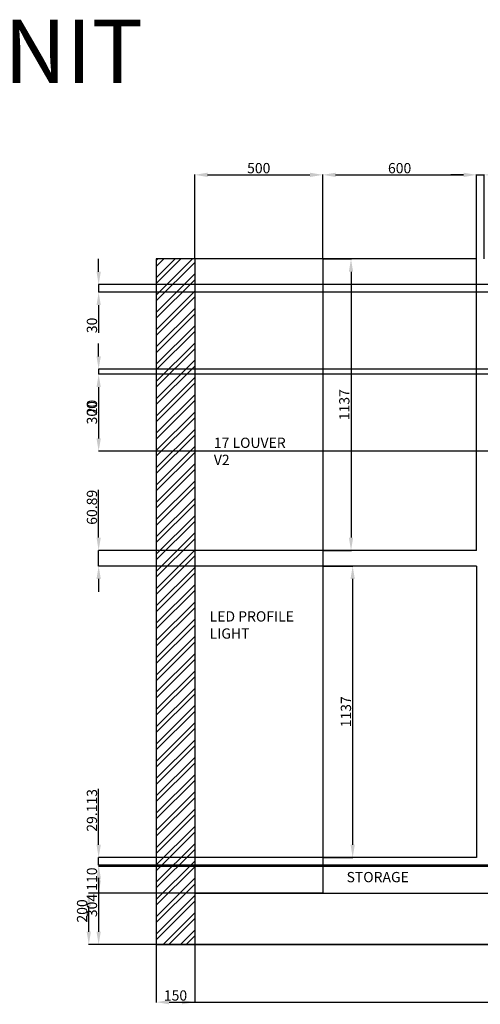
# Model space of a CAD drawing. Units: millimetres. Extents: x -2182 to 7969, y 257 to 4097.
# Tile 3 of 5: x 2894 to 4692, y 257 to 4097. Entities that reach past the tile are written whole.
import ezdxf

# ---------------------------------------------------------------- set-up
doc = ezdxf.new("R2010")
doc.units = ezdxf.units.MM
for name, color, linetype, lineweight in [('A-ANNO-DIMS', 2, 'Continuous', 18), ('A-ANNO-TEXT', 3, 'Continuous', 18), ('A-ELEV', 7, 'Continuous', 25), ('A-ELEV-PATT', 8, 'Continuous', 13)]:
    doc.layers.add(name, color=color, linetype=linetype, lineweight=lineweight)
doc.styles.get("Standard").update_dxf_attribs({"font": 'arial.ttf'})
doc.dimstyles.new('ISO-25', dxfattribs={"dimtxt": 40, "dimasz": 50, "dimexe": 1.25, "dimexo": 0.625, "dimtad": 1, "dimtxsty": 'Standard', "dimcen": 2.5, "dimadec": 0, "dimazin": 0, "dimtfac": 1, "dimtmove": 0, "dimatfit": 3, "dimfxl": 1, "dimarcsym": 0})

# ---------------------------------------------------------------- blocks, each defined once
blk = doc.blocks.new('*D34')
at = {"layer": 'A-ANNO-DIMS', "color": 0, "lineweight": -2, "transparency": 16777216}
for p, q in [((4077.6, 3164), (4188.4, 3164)), ((4187.1, 3114), (4187.1, 2077)), ((4077.6, 2027), (4188.4, 2027))]:
    blk.add_line(p, q, dxfattribs=at)
at = {"layer": 'A-ANNO-DIMS', "color": 0, "transparency": 16777216}
for points in [[(4178.8, 3114), (4195.5, 3114), (4187.1, 3164)], [(4178.8, 2077), (4195.5, 2077), (4187.1, 2027)]]:
    blk.add_solid(points, dxfattribs=at)
at = {"layer": 'Defpoints', "color": 0, "transparency": 16777216}
for p in [(4076.9, 3164), (4076.9, 2027), (4187.1, 2027)]:
    blk.add_point(p, dxfattribs=at)
at = {"layer": 'A-ANNO-DIMS', "color": 0, "transparency": 16777216, "insert": (4166.1, 2595.5), "char_height": 40, "attachment_point": 5, "rotation": 90}
blk.add_mtext('1137', dxfattribs=at)
blk = doc.blocks.new('*D35')
at = {"layer": 'A-ANNO-DIMS', "color": 0, "lineweight": -2, "transparency": 16777216}
for p, q in [((4077.6, 1966.1), (4194.8, 1966.1)), ((4193.6, 879.1), (4193.6, 1916.1)), ((4077.6, 829.1), (4194.8, 829.1))]:
    blk.add_line(p, q, dxfattribs=at)
at = {"layer": 'A-ANNO-DIMS', "color": 0, "transparency": 16777216}
for points in [[(4185.3, 1916.1), (4201.9, 1916.1), (4193.6, 1966.1)], [(4185.3, 879.1), (4201.9, 879.1), (4193.6, 829.1)]]:
    blk.add_solid(points, dxfattribs=at)
at = {"layer": 'Defpoints', "color": 0, "transparency": 16777216}
for p in [(4076.9, 1966.1), (4193.6, 1966.1), (4076.9, 829.1)]:
    blk.add_point(p, dxfattribs=at)
at = {"layer": 'A-ANNO-DIMS', "color": 0, "transparency": 16777216, "insert": (4172.5, 1397.6), "char_height": 40, "attachment_point": 5, "rotation": 90}
blk.add_mtext('1137', dxfattribs=at)
blk = doc.blocks.new('*D36')
at = {"layer": 'A-ANNO-DIMS', "color": 0, "lineweight": -2, "transparency": 16777216}
for p, q in [((3426.3, 690), (3162.1, 690)), ((3163.4, 540), (3163.4, 640)), ((3426.3, 490), (3162.1, 490))]:
    blk.add_line(p, q, dxfattribs=at)
at = {"layer": 'A-ANNO-DIMS', "color": 0, "transparency": 16777216}
for points in [[(3155, 640), (3171.7, 640), (3163.4, 690)], [(3155, 540), (3171.7, 540), (3163.4, 490)]]:
    blk.add_solid(points, dxfattribs=at)
at = {"layer": 'Defpoints', "color": 0, "transparency": 16777216}
for p in [(3163.4, 690), (3426.9, 690), (3426.9, 490)]:
    blk.add_point(p, dxfattribs=at)
at = {"layer": 'A-ANNO-DIMS', "color": 0, "transparency": 16777216, "insert": (3142.3, 620.8), "char_height": 40, "attachment_point": 5, "rotation": 90}
blk.add_mtext('200', dxfattribs=at)
blk = doc.blocks.new('*D77')
at = {"layer": 'A-ANNO-DIMS', "color": 0, "lineweight": -2, "transparency": 16777216}
for p, q in [((7735.9, 3063.4), (7735.9, 263.7)), ((3426.9, 489.4), (3426.9, 263.7)), ((3476.9, 265), (7685.9, 265))]:
    blk.add_line(p, q, dxfattribs=at)
at = {"layer": 'A-ANNO-DIMS', "color": 0, "transparency": 16777216}
for points in [[(3476.9, 273.3), (3476.9, 256.7), (3426.9, 265)], [(7685.9, 273.3), (7685.9, 256.7), (7735.9, 265)]]:
    blk.add_solid(points, dxfattribs=at)
at = {"layer": 'Defpoints', "color": 0, "transparency": 16777216}
for p in [(7735.9, 3064), (3426.9, 490), (7735.9, 265)]:
    blk.add_point(p, dxfattribs=at)
at = {"layer": 'A-ANNO-DIMS', "color": 0, "transparency": 16777216, "insert": (5581.4, 286.1), "char_height": 40, "attachment_point": 5}
blk.add_mtext('4309', dxfattribs=at)
blk = doc.blocks.new('*D78')
at = {"layer": 'A-ANNO-DIMS', "color": 0, "lineweight": -2, "transparency": 16777216}
for p, q in [((3426.9, 489.4), (3426.9, 263.7)), ((3576.9, 489.4), (3576.9, 263.7)), ((3476.9, 265), (3526.9, 265))]:
    blk.add_line(p, q, dxfattribs=at)
at = {"layer": 'A-ANNO-DIMS', "color": 0, "transparency": 16777216}
for points in [[(3476.9, 273.3), (3476.9, 256.7), (3426.9, 265)], [(3526.9, 273.3), (3526.9, 256.7), (3576.9, 265)]]:
    blk.add_solid(points, dxfattribs=at)
at = {"layer": 'Defpoints', "color": 0, "transparency": 16777216}
for p in [(3426.9, 490), (3576.9, 490), (3576.9, 265)]:
    blk.add_point(p, dxfattribs=at)
at = {"layer": 'A-ANNO-DIMS', "color": 0, "transparency": 16777216, "insert": (3501.9, 286), "char_height": 40, "attachment_point": 5}
blk.add_mtext('150', dxfattribs=at)
blk = doc.blocks.new('*D79')
at = {"layer": 'A-ANNO-DIMS', "color": 0, "lineweight": -2, "transparency": 16777216}
for p, q in [((7736.6, 3164), (7962.2, 3164)), ((7960.9, 3114), (7960.9, 540)), ((3427.6, 490), (7962.2, 490))]:
    blk.add_line(p, q, dxfattribs=at)
at = {"layer": 'A-ANNO-DIMS', "color": 0, "transparency": 16777216}
for points in [[(7952.6, 3114), (7969.3, 3114), (7960.9, 3164)], [(7952.6, 540), (7969.3, 540), (7960.9, 490)]]:
    blk.add_solid(points, dxfattribs=at)
at = {"layer": 'Defpoints', "color": 0, "transparency": 16777216}
for p in [(7735.9, 3164), (3426.9, 490), (7960.9, 490)]:
    blk.add_point(p, dxfattribs=at)
at = {"layer": 'A-ANNO-DIMS', "color": 0, "transparency": 16777216, "insert": (7939.9, 1827), "char_height": 40, "attachment_point": 5, "rotation": 90}
blk.add_mtext('2674', dxfattribs=at)
blk = doc.blocks.new('*D80')
at = {"layer": 'A-ANNO-DIMS', "color": 0, "lineweight": -2, "transparency": 16777216}
for p, q in [((3576.9, 3164.6), (3576.9, 3493.3)), ((3626.9, 3492), (4026.9, 3492)), ((4076.9, 3164.6), (4076.9, 3493.3))]:
    blk.add_line(p, q, dxfattribs=at)
at = {"layer": 'A-ANNO-DIMS', "color": 0, "transparency": 16777216}
for points in [[(3626.9, 3500.4), (3626.9, 3483.7), (3576.9, 3492)], [(4026.9, 3500.4), (4026.9, 3483.7), (4076.9, 3492)]]:
    blk.add_solid(points, dxfattribs=at)
at = {"layer": 'Defpoints', "color": 0, "transparency": 16777216}
for p in [(4076.9, 3492), (3576.9, 3164), (4076.9, 3164)]:
    blk.add_point(p, dxfattribs=at)
at = {"layer": 'A-ANNO-DIMS', "color": 0, "transparency": 16777216, "insert": (3826.9, 3513.1), "char_height": 40, "attachment_point": 5}
blk.add_mtext('500', dxfattribs=at)
blk = doc.blocks.new('*D81')
at = {"layer": 'A-ANNO-DIMS', "color": 0, "lineweight": -2, "transparency": 16777216}
for p, q in [((4076.9, 3164.6), (4076.9, 3493.3)), ((4126.9, 3492), (4626.9, 3492)), ((4676.9, 3164.6), (4676.9, 3493.3))]:
    blk.add_line(p, q, dxfattribs=at)
at = {"layer": 'A-ANNO-DIMS', "color": 0, "transparency": 16777216}
for points in [[(4126.9, 3500.4), (4126.9, 3483.7), (4076.9, 3492)], [(4626.9, 3500.4), (4626.9, 3483.7), (4676.9, 3492)]]:
    blk.add_solid(points, dxfattribs=at)
at = {"layer": 'Defpoints', "color": 0, "transparency": 16777216}
for p in [(4676.9, 3492), (4076.9, 3164), (4676.9, 3164)]:
    blk.add_point(p, dxfattribs=at)
at = {"layer": 'A-ANNO-DIMS', "color": 0, "transparency": 16777216, "insert": (4376.9, 3513.1), "char_height": 40, "attachment_point": 5}
blk.add_mtext('600', dxfattribs=at)
blk = doc.blocks.new('*D82')
at = {"layer": 'A-ANNO-DIMS', "color": 0, "lineweight": -2, "transparency": 16777216}
for p, q in [((4626.9, 3492), (4576.9, 3492)), ((4676.9, 3164.6), (4676.9, 3493.3)), ((4676.9, 3492), (4706.9, 3492)), ((4706.9, 3164.6), (4706.9, 3493.3)), ((4756.9, 3492), (4865.3, 3492))]:
    blk.add_line(p, q, dxfattribs=at)
at = {"layer": 'A-ANNO-DIMS', "color": 0, "transparency": 16777216}
for points in [[(4626.9, 3500.4), (4626.9, 3483.7), (4676.9, 3492)], [(4756.9, 3500.4), (4756.9, 3483.7), (4706.9, 3492)]]:
    blk.add_solid(points, dxfattribs=at)
at = {"layer": 'Defpoints', "color": 0, "transparency": 16777216}
for p in [(4706.9, 3492), (4676.9, 3164), (4706.9, 3164)]:
    blk.add_point(p, dxfattribs=at)
at = {"layer": 'A-ANNO-DIMS', "color": 0, "transparency": 16777216, "insert": (4836.1, 3513.1), "char_height": 40, "attachment_point": 5}
blk.add_mtext('30', dxfattribs=at)
blk = doc.blocks.new('*D85')
at = {"layer": 'A-ANNO-DIMS', "color": 0, "lineweight": -2, "transparency": 16777216}
for p, q in [((4076.3, 800), (3200.7, 800)), ((3201.9, 740), (3201.9, 750)), ((4076.3, 690), (3200.7, 690))]:
    blk.add_line(p, q, dxfattribs=at)
at = {"layer": 'A-ANNO-DIMS', "color": 0, "transparency": 16777216}
for points in [[(3193.6, 750), (3210.3, 750), (3201.9, 800)], [(3193.6, 740), (3210.3, 740), (3201.9, 690)]]:
    blk.add_solid(points, dxfattribs=at)
at = {"layer": 'Defpoints', "color": 0, "transparency": 16777216}
for p in [(3201.9, 800), (4076.9, 800), (4076.9, 690)]:
    blk.add_point(p, dxfattribs=at)
at = {"layer": 'A-ANNO-DIMS', "color": 0, "transparency": 16777216, "insert": (3180.9, 745), "char_height": 40, "attachment_point": 5, "rotation": 90}
blk.add_mtext('110', dxfattribs=at)
blk = doc.blocks.new('*D86')
at = {"layer": 'A-ANNO-DIMS', "color": 0, "lineweight": -2, "transparency": 16777216}
for p, q in [((3201.9, 879.1), (3201.9, 1097.1)), ((4076.3, 829.1), (3200.7, 829.1)), ((3201.9, 800), (3201.9, 829.1)), ((4076.3, 800), (3200.7, 800)), ((3201.9, 750), (3201.9, 700))]:
    blk.add_line(p, q, dxfattribs=at)
at = {"layer": 'A-ANNO-DIMS', "color": 0, "transparency": 16777216}
for points in [[(3193.6, 879.1), (3210.3, 879.1), (3201.9, 829.1)], [(3193.6, 750), (3210.3, 750), (3201.9, 800)]]:
    blk.add_solid(points, dxfattribs=at)
at = {"layer": 'Defpoints', "color": 0, "transparency": 16777216}
for p in [(3201.9, 829.1), (4076.9, 829.1), (4076.9, 800)]:
    blk.add_point(p, dxfattribs=at)
at = {"layer": 'A-ANNO-DIMS', "color": 0, "transparency": 16777216, "insert": (3180.9, 1013.1), "char_height": 40, "attachment_point": 5, "rotation": 90}
blk.add_mtext('29.113', dxfattribs=at)
blk = doc.blocks.new('*D87')
at = {"layer": 'A-ANNO-DIMS', "color": 0, "lineweight": -2, "transparency": 16777216}
for p, q in [((3201.9, 2077), (3201.9, 2263.5)), ((4076.3, 2027), (3200.7, 2027)), ((3201.9, 1966.1), (3201.9, 2027)), ((4076.3, 1966.1), (3200.7, 1966.1)), ((3201.9, 1916.1), (3201.9, 1866.1))]:
    blk.add_line(p, q, dxfattribs=at)
at = {"layer": 'A-ANNO-DIMS', "color": 0, "transparency": 16777216}
for points in [[(3193.6, 2077), (3210.3, 2077), (3201.9, 2027)], [(3193.6, 1916.1), (3210.3, 1916.1), (3201.9, 1966.1)]]:
    blk.add_solid(points, dxfattribs=at)
at = {"layer": 'Defpoints', "color": 0, "transparency": 16777216}
for p in [(3201.9, 2027), (4076.9, 2027), (4076.9, 1966.1)]:
    blk.add_point(p, dxfattribs=at)
at = {"layer": 'A-ANNO-DIMS', "color": 0, "transparency": 16777216, "insert": (3180.9, 2195.3), "char_height": 40, "attachment_point": 5, "rotation": 90}
blk.add_mtext('60.89', dxfattribs=at)
blk = doc.blocks.new('*D92')
at = {"layer": 'A-ANNO-DIMS', "color": 0, "lineweight": -2, "transparency": 16777216}
for p, q in [((3201.9, 3114), (3201.9, 3164)), ((6585.3, 3064), (3200.7, 3064)), ((3201.9, 3064), (3201.9, 3034)), ((6615.3, 3034), (3200.7, 3034)), ((3201.9, 2984), (3201.9, 2875.6))]:
    blk.add_line(p, q, dxfattribs=at)
at = {"layer": 'A-ANNO-DIMS', "color": 0, "transparency": 16777216}
for points in [[(3193.6, 3114), (3210.3, 3114), (3201.9, 3064)], [(3193.6, 2984), (3210.3, 2984), (3201.9, 3034)]]:
    blk.add_solid(points, dxfattribs=at)
at = {"layer": 'Defpoints', "color": 0, "transparency": 16777216}
for p in [(6585.9, 3064), (3201.9, 3034), (6615.9, 3034)]:
    blk.add_point(p, dxfattribs=at)
at = {"layer": 'A-ANNO-DIMS', "color": 0, "transparency": 16777216, "insert": (3180.9, 2904.8), "char_height": 40, "attachment_point": 5, "rotation": 90}
blk.add_mtext('30', dxfattribs=at)
blk = doc.blocks.new('*D93')
at = {"layer": 'A-ANNO-DIMS', "color": 0, "lineweight": -2, "transparency": 16777216}
for p, q in [((3201.9, 2784), (3201.9, 2834)), ((6615.3, 2734), (3200.7, 2734)), ((3201.9, 2734), (3201.9, 2714)), ((6615.3, 2714), (3200.7, 2714)), ((3201.9, 2664), (3201.9, 2554.9))]:
    blk.add_line(p, q, dxfattribs=at)
at = {"layer": 'A-ANNO-DIMS', "color": 0, "transparency": 16777216}
for points in [[(3193.6, 2784), (3210.3, 2784), (3201.9, 2734)], [(3193.6, 2664), (3210.3, 2664), (3201.9, 2714)]]:
    blk.add_solid(points, dxfattribs=at)
at = {"layer": 'Defpoints', "color": 0, "transparency": 16777216}
for p in [(6615.9, 2734), (3201.9, 2714), (6615.9, 2714)]:
    blk.add_point(p, dxfattribs=at)
at = {"layer": 'A-ANNO-DIMS', "color": 0, "transparency": 16777216, "insert": (3180.9, 2584.4), "char_height": 40, "attachment_point": 5, "rotation": 90}
blk.add_mtext('20', dxfattribs=at)
blk = doc.blocks.new('*D94')
at = {"layer": 'A-ANNO-DIMS', "color": 0, "lineweight": -2, "transparency": 16777216}
for p, q in [((6615.3, 2714), (3200.7, 2714)), ((3201.9, 2664), (3201.9, 2464)), ((6615.3, 2414), (3200.7, 2414))]:
    blk.add_line(p, q, dxfattribs=at)
at = {"layer": 'A-ANNO-DIMS', "color": 0, "transparency": 16777216}
for points in [[(3193.6, 2664), (3210.3, 2664), (3201.9, 2714)], [(3193.6, 2464), (3210.3, 2464), (3201.9, 2414)]]:
    blk.add_solid(points, dxfattribs=at)
at = {"layer": 'Defpoints', "color": 0, "transparency": 16777216}
for p in [(6615.9, 2714), (3201.9, 2414), (6615.9, 2414)]:
    blk.add_point(p, dxfattribs=at)
at = {"layer": 'A-ANNO-DIMS', "color": 0, "transparency": 16777216, "insert": (3180.9, 2564), "char_height": 40, "attachment_point": 5, "rotation": 90}
blk.add_mtext('300', dxfattribs=at)
blk = doc.blocks.new('*D95')
at = {"layer": 'A-ANNO-DIMS', "color": 0, "lineweight": -2, "transparency": 16777216}
for p, q in [((6615.3, 794), (3200.7, 794)), ((3201.9, 744), (3201.9, 540)), ((6615.3, 490), (3200.7, 490))]:
    blk.add_line(p, q, dxfattribs=at)
at = {"layer": 'A-ANNO-DIMS', "color": 0, "transparency": 16777216}
for points in [[(3193.6, 744), (3210.3, 744), (3201.9, 794)], [(3193.6, 540), (3210.3, 540), (3201.9, 490)]]:
    blk.add_solid(points, dxfattribs=at)
at = {"layer": 'Defpoints', "color": 0, "transparency": 16777216}
for p in [(6615.9, 794), (3201.9, 490), (6615.9, 490)]:
    blk.add_point(p, dxfattribs=at)
at = {"layer": 'A-ANNO-DIMS', "color": 0, "transparency": 16777216, "insert": (3180.9, 642), "char_height": 40, "attachment_point": 5, "rotation": 90}
blk.add_mtext('304', dxfattribs=at)

msp = doc.modelspace()

# ---------------------------------------------------------------- hatches: boundary and pattern name
at = {"layer": 'A-ELEV-PATT'}
h = msp.add_hatch(dxfattribs=at)
h.set_pattern_fill('ANSI32', color=256, scale=5)
h.paths.add_polyline_path([(3576.9478, 3163.9911), (3426.9478, 3163.9911), (3426.9478, 489.9911), (3576.9478, 489.9911)])

# ---------------------------------------------------------------- linework, layer by layer
at = {"layer": 'A-ELEV'}
for p, q in [((4676.9478, 3163.9911), (3426.9478, 3163.9911)), ((3426.9478, 3163.9911), (3426.9478, 489.9911)), ((3576.9478, 3163.9911), (3576.9478, 489.9911)), ((4076.9478, 3163.9911), (4076.9478, 689.9911)), ((4676.9478, 2026.9911), (4676.9478, 3163.9911)), ((4676.9478, 2026.9911), (4076.9478, 2026.9911)), ((4676.9478, 1966.1042), (4076.9478, 1966.1042)), ((4676.9478, 1966.1042), (4676.9478, 829.1042)), ((4676.9478, 829.1042), (4076.9478, 829.1042)), ((6585.9478, 799.9911), (4076.9478, 799.9911)), ((3576.9478, 689.9911), (6585.9478, 689.9911)), ((3426.9478, 489.9911), (7685.9478, 489.9911))]:
    msp.add_line(p, q, dxfattribs=at)

# ---------------------------------------------------------------- texts
at = {"layer": 'A-ANNO-TEXT', "attachment_point": 1}
for s, insert, char_height, width in [('TV UNIT ', (2120.501, 4097.2574), 246.35353, 3842.081942), ('17 LOUVER \\P     V2', (3651.613, 2466.9142), 40, 482.986246), ('LED PROFILE \\PLIGHT', (3635.2059, 1789.6743), 40, 482.986246), ('STORAGE', (4169.7322, 772.8904), 40, 482.986246)]:
    msp.add_mtext(s, dxfattribs=dict(at, insert=insert, char_height=char_height, width=width))

# ---------------------------------------------------------------- dimensions: what is measured, and where the dimension line sits
at = {"layer": 'A-ANNO-DIMS'}
for base, p1, p2, picture, middle in [((4076.9478, 3492.0268), (3576.9478, 3163.9911), (4076.9478, 3163.9911), '*D80', (3826.9478, 3513.0747)), ((4676.9478, 3492.0268), (4076.9478, 3163.9911), (4676.9478, 3163.9911), '*D81', (4376.9478, 3513.0747)), ((4706.9478, 3492.0268), (4676.9478, 3163.9911), (4706.9478, 3163.9911), '*D82', (4836.1403, 3513.0883)), ((7735.9478, 264.9911), (3426.9478, 489.9911), (7735.9478, 3063.9911), '*D77', (5581.4478, 286.0526)), ((3576.9478, 264.9911), (3426.9478, 489.9911), (3576.9478, 489.9911), '*D78', (3501.9478, 286.039))]:
    dim = msp.add_linear_dim(base=base, p1=p1, p2=p2, dimstyle='ISO-25', override={"dimdec": 0, "dimlfac": 1, "dimrnd": 0, "dimzin": 0, "dimdsep": 46, "dimlunit": 2}, dxfattribs=at)
    dim.commit()
    dim.dimension.update_dxf_attribs({"geometry": picture, "text_midpoint": middle})
for base, p1, p2, override, picture, middle in [((3201.9478, 3033.9911), (6585.9478, 3063.9911), (6615.9478, 3033.9911), {"dimdec": 0, "dimlfac": 1, "dimrnd": 0, "dimzin": 0, "dimdsep": 46, "dimlunit": 2}, '*D92', (3180.8862, 2904.7985)), ((7960.9478, 489.9911), (7735.9478, 3163.9911), (3426.9478, 489.9911), {"dimdec": 0, "dimlfac": 1, "dimrnd": 0, "dimzin": 0, "dimdsep": 46, "dimlunit": 2}, '*D79', (7939.8999, 1826.9911)), ((4187.1308, 2026.9911), (4076.9478, 3163.9911), (4076.9478, 2026.9911), {"dimclrd": 0, "dimclre": 0, "dimclrt": 0}, '*D34', (4166.0693, 2595.4911)), ((3201.9478, 2713.9911), (6615.9478, 2733.9911), (6615.9478, 2713.9911), {"dimdec": 0, "dimlfac": 1, "dimrnd": 0, "dimzin": 0, "dimdsep": 46, "dimlunit": 2}, '*D93', (3180.8999, 2584.4438)), ((3201.9478, 2413.9911), (6615.9478, 2713.9911), (6615.9478, 2413.9911), {"dimdec": 0, "dimlfac": 1, "dimrnd": 0, "dimzin": 0, "dimdsep": 46, "dimlunit": 2}, '*D94', (3180.8862, 2563.9911)), ((3201.9478, 2026.9911), (4076.9478, 1966.1042), (4076.9478, 2026.9911), {"dimdec": 2, "dimlfac": 1, "dimrnd": 0, "dimzin": 0, "dimdsep": 46, "dimlunit": 2}, '*D87', (3180.8999, 2195.2559)), ((4193.5992, 1966.1042), (4076.9478, 829.1042), (4076.9478, 1966.1042), {"dimclrd": 0, "dimclre": 0, "dimclrt": 0}, '*D35', (4172.5377, 1397.6042)), ((3201.9478, 829.1042), (4076.9478, 799.9911), (4076.9478, 829.1042), {"dimdec": 3, "dimlfac": 1, "dimrnd": 0, "dimzin": 0, "dimdsep": 46, "dimlunit": 2}, '*D86', (3180.8862, 1013.0989)), ((3201.9478, 489.9911), (6615.9478, 793.9911), (6615.9478, 489.9911), {"dimdec": 0, "dimlfac": 1, "dimrnd": 0, "dimzin": 0, "dimdsep": 46, "dimlunit": 2}, '*D95', (3180.8862, 641.9911)), ((3201.9478, 799.9911), (4076.9478, 689.9911), (4076.9478, 799.9911), {"dimdec": 0, "dimlfac": 1, "dimrnd": 0, "dimzin": 0, "dimdsep": 46, "dimlunit": 2}, '*D85', (3180.8999, 744.9911))]:
    dim = msp.add_linear_dim(base=base, p1=p1, p2=p2, angle=90, dimstyle='ISO-25', override=override, dxfattribs=at)
    dim.commit()
    dim.dimension.update_dxf_attribs({"geometry": picture, "text_midpoint": middle})
dim = msp.add_linear_dim(base=(3163.3513, 689.9911), p1=(3426.9478, 489.9911), p2=(3426.9478, 689.9911), angle=90, dimstyle='ISO-25', override={"dimclrd": 0, "dimclre": 0, "dimclrt": 0}, dxfattribs=at)
dim.commit()
dim.dimension.update_dxf_attribs({"geometry": '*D36', "text_midpoint": (3163.3513, 620.7667), "dimtype": 160})

doc.saveas('drawing.dxf')
